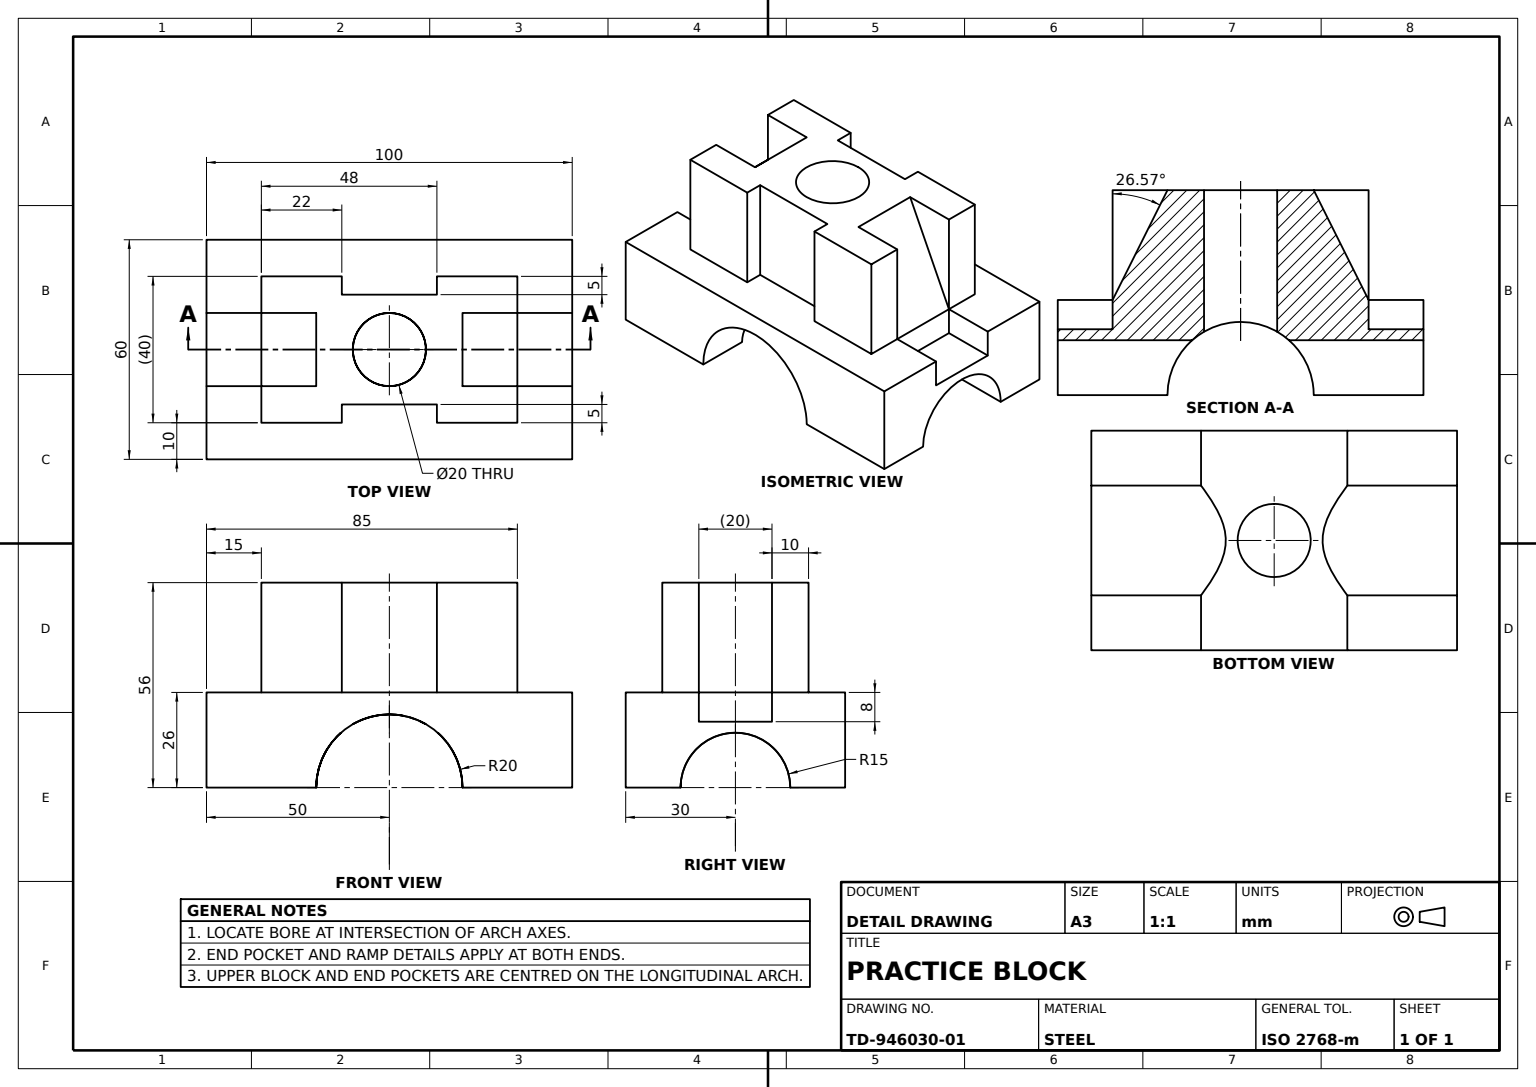
from build123d import *

# Parameters (mm, degrees)
BASE_BLOCK_DEPTH        = 26
UPPER_GUIDE_BLOCK_DEPTH = 30
GUIDE_SLOTS_SKETCH_W    = 26
GUIDE_SLOTS_SKETCH_H    = 5
GUIDE_SLOTS_SKETCH_W_2  = 15
GUIDE_SLOTS_SKETCH_H_2  = 20
GUIDE_SLOTS_CUT_DEPTH   = 30
OFFSET_BOSS_DEPTH       = 20
TOP_BORE_SKETCH_R       = 10
TOP_BORE_DEPTH          = 83
POCKET_SKETCH_W         = 15
POCKET_SKETCH_H         = 20
POCKET_8MM_DEEP_DEPTH   = 8
SIDE_ARCH_CUT_DEPTH     = 121
BEARING_ARCH_SKETCH_R   = 20
BEARING_ARCH_CUT_DEPTH  = 121


with BuildPart() as part:
    # Base Profile Sketch → Base Block (new body)
    with BuildSketch(Plane(origin=(0, 0, 0), x_dir=(1, 0, 0), z_dir=(0, 1, 0))):
        Polygon((50, 0), (50, 30), (-50, 30), (-50, -30), (50, -30), align=None)
    extrude(amount=BASE_BLOCK_DEPTH)

    # Upper Block Sketch → Upper Guide Block (add)
    with BuildSketch(Plane(origin=(0, 26, 0), x_dir=(1, 0, 0), z_dir=(0, 1, 0))):
        Polygon((35, 0), (35, 20), (-35, 20), (-35, -20), (35, -20), align=None)
    extrude(amount=UPPER_GUIDE_BLOCK_DEPTH)

    # Guide Slots Sketch → Guide Slots Cut (cut)
    with BuildSketch(Plane(origin=(0, 56, 0), x_dir=(1, 0, 0), z_dir=(0, 1, 0))):
        Polygon((35, 0), (35, 10), (20, 10), (20, -10), (35, -10), align=None)
        with Locations((0, -17.5)):
            Rectangle(GUIDE_SLOTS_SKETCH_W, GUIDE_SLOTS_SKETCH_H)
        with Locations((-27.5, 0)):
            Rectangle(GUIDE_SLOTS_SKETCH_W_2, GUIDE_SLOTS_SKETCH_H_2)
        with Locations((0, 17.5)):
            Rectangle(GUIDE_SLOTS_SKETCH_W, GUIDE_SLOTS_SKETCH_H)
    extrude(amount=-GUIDE_SLOTS_CUT_DEPTH, mode=Mode.SUBTRACT)

    # Offset Boss Sketch → Offset Boss (add)
    with BuildSketch(Plane.XY.offset(10)):
        Polygon((-20, 56), (-35, 26), (-20, 26), align=None)
        Polygon((20, 56), (35, 26), (20, 26), align=None)
    extrude(amount=-OFFSET_BOSS_DEPTH)

    # Top Bore Sketch → Top Bore (cut)
    with BuildSketch(Plane(origin=(0, 56, 0), x_dir=(1, 0, 0), z_dir=(0, 1, 0))):
        with Locations(Location((0, 0, 0), (0, 0, 270))):
            Circle(TOP_BORE_SKETCH_R)
    extrude(amount=-TOP_BORE_DEPTH, mode=Mode.SUBTRACT)

    # Pocket Sketch → Pocket 8mm Deep (cut)
    with BuildSketch(Plane(origin=(0, 26, 0), x_dir=(1, 0, 0), z_dir=(0, 1, 0))):
        with Locations((42.5, 0)):
            Rectangle(POCKET_SKETCH_W, POCKET_SKETCH_H)
        with Locations((-42.5, 0)):
            Rectangle(POCKET_SKETCH_W, POCKET_SKETCH_H)
    extrude(amount=-POCKET_8MM_DEEP_DEPTH, mode=Mode.SUBTRACT)

    # Side Arch Sketch → Side Arch Cut (cut)
    with BuildSketch(Plane.ZY.offset(50)):
        with BuildLine():
            Line((-15, 0), (15, 0))
            ThreePointArc((15, 0), (0, 15), (-15, 0))
        make_face()
    extrude(amount=-SIDE_ARCH_CUT_DEPTH, mode=Mode.SUBTRACT)

    # Bearing Arch Sketch → Bearing Arch Cut (cut)
    with BuildSketch(Plane(origin=(0, 0, -30), x_dir=(-1, 0, 0), z_dir=(0, 0, -1))):
        Circle(BEARING_ARCH_SKETCH_R)
    extrude(amount=-BEARING_ARCH_CUT_DEPTH, mode=Mode.SUBTRACT)


solid = part.part
